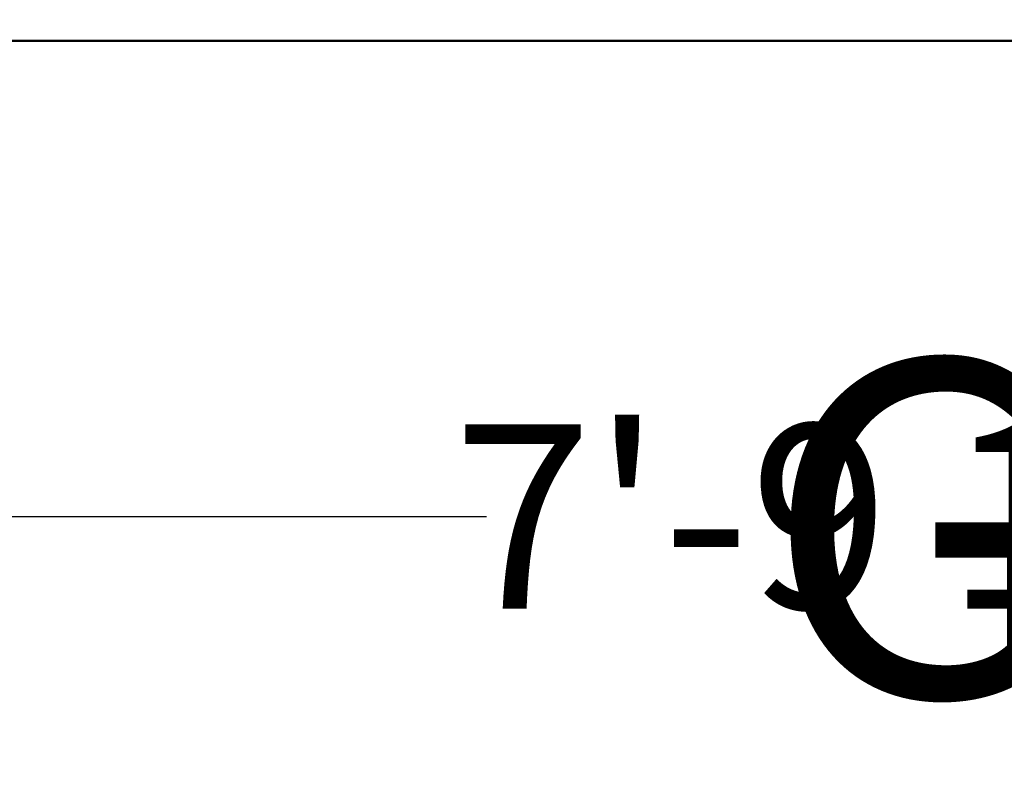
# Model space of a CAD drawing. Units: inches. Extents: x 22042254 to 25404563, y 17568978 to 17626777.
# Tile 20 of 45: x 22179809 to 22179852, y 17626160 to 17626194. Entities that reach past the tile are written whole.
import ezdxf

# ---------------------------------------------------------------- set-up
doc = ezdxf.new("R2010")
doc.units = ezdxf.units.IN
doc.header["$MEASUREMENT"] = 0
for name, color, linetype, lineweight in [('A-ANNO-DIMS', 2, 'Continuous', 18), ('text', 7, 'Continuous', 25), ('walls', 252, 'Continuous', 50)]:
    doc.layers.add(name, color=color, linetype=linetype, lineweight=lineweight)
doc.styles.get("Standard").update_dxf_attribs({"font": 'arial.ttf'})
doc.dimstyles.get("Standard").update_dxf_attribs({"dimtxt": 8, "dimasz": 0.18, "dimexe": 0.18, "dimexo": 0.0625, "dimgap": 0.09, "dimtad": 0, "dimtih": 1, "dimtoh": 1, "dimzin": 0, "dimdsep": 46, "dimlunit": 3, "dimtxsty": 'Standard', "dimcen": 0.09, "dimadec": 0, "dimazin": 0, "dimtfac": 1, "dimtofl": 0, "dimtmove": 0, "dimatfit": 3, "dimfxl": 1, "dimtolj": 1, "dimtzin": 0, "dimarcsym": 0})

# ---------------------------------------------------------------- blocks, each defined once
blk = doc.blocks.new('*D59')
at = {"layer": 'A-ANNO-DIMS', "color": 0, "lineweight": -2, "transparency": 16777216}
for p, q in [((22179802.402, 17626200.497), (22179802.402, 17626171.756)), ((22179895.926, 17626200.497), (22179895.926, 17626171.756)), ((22179802.582, 17626171.936), (22179829.153, 17626171.936)), ((22179895.746, 17626171.936), (22179869.175, 17626171.936))]:
    blk.add_line(p, q, dxfattribs=at)
at = {"layer": 'A-ANNO-DIMS', "color": 0, "transparency": 16777216}
for points in [[(22179802.582, 17626171.966), (22179802.582, 17626171.906), (22179802.402, 17626171.936)], [(22179895.746, 17626171.966), (22179895.746, 17626171.906), (22179895.926, 17626171.936)]]:
    blk.add_solid(points, dxfattribs=at)
at = {"layer": 'Defpoints', "color": 0, "transparency": 16777216}
for p in [(22179802.402, 17626200.559), (22179895.926, 17626200.559), (22179895.926, 17626171.936)]:
    blk.add_point(p, dxfattribs=at)
at = {"layer": 'A-ANNO-DIMS', "color": 0, "transparency": 16777216, "insert": (22179849.164, 17626171.936), "char_height": 8, "attachment_point": 5}
blk.add_mtext('\\A1;7\'-9 1/2"', dxfattribs=at)

msp = doc.modelspace()

# ---------------------------------------------------------------- linework, layer by layer
at = {"layer": 'walls'}
msp.add_line((22179783.734, 17626192.584), (22179936.734, 17626192.584), dxfattribs=at)

# ---------------------------------------------------------------- texts
at = {"layer": 'text'}
msp.add_text('GROUND FLOOR PLAN', height=14.58777, dxfattribs=at).set_placement((22179841.196, 17626164.124))

# ---------------------------------------------------------------- dimensions: what is measured, and where the dimension line sits
at = {"layer": 'A-ANNO-DIMS'}
dim = msp.add_linear_dim(base=(22179895.926, 17626171.936), p1=(22179802.402, 17626200.559), p2=(22179895.926, 17626200.559), dimstyle='Standard', override={"dimdec": 1, "dimlfac": 1, "dimrnd": 0, "dimzin": 1, "dimdsep": 46, "dimlunit": 4, "dimfrac": 2}, dxfattribs=at)
dim.commit()
dim.dimension.update_dxf_attribs({"geometry": '*D59', "text_midpoint": (22179849.164, 17626171.936)})

doc.saveas('drawing.dxf')
